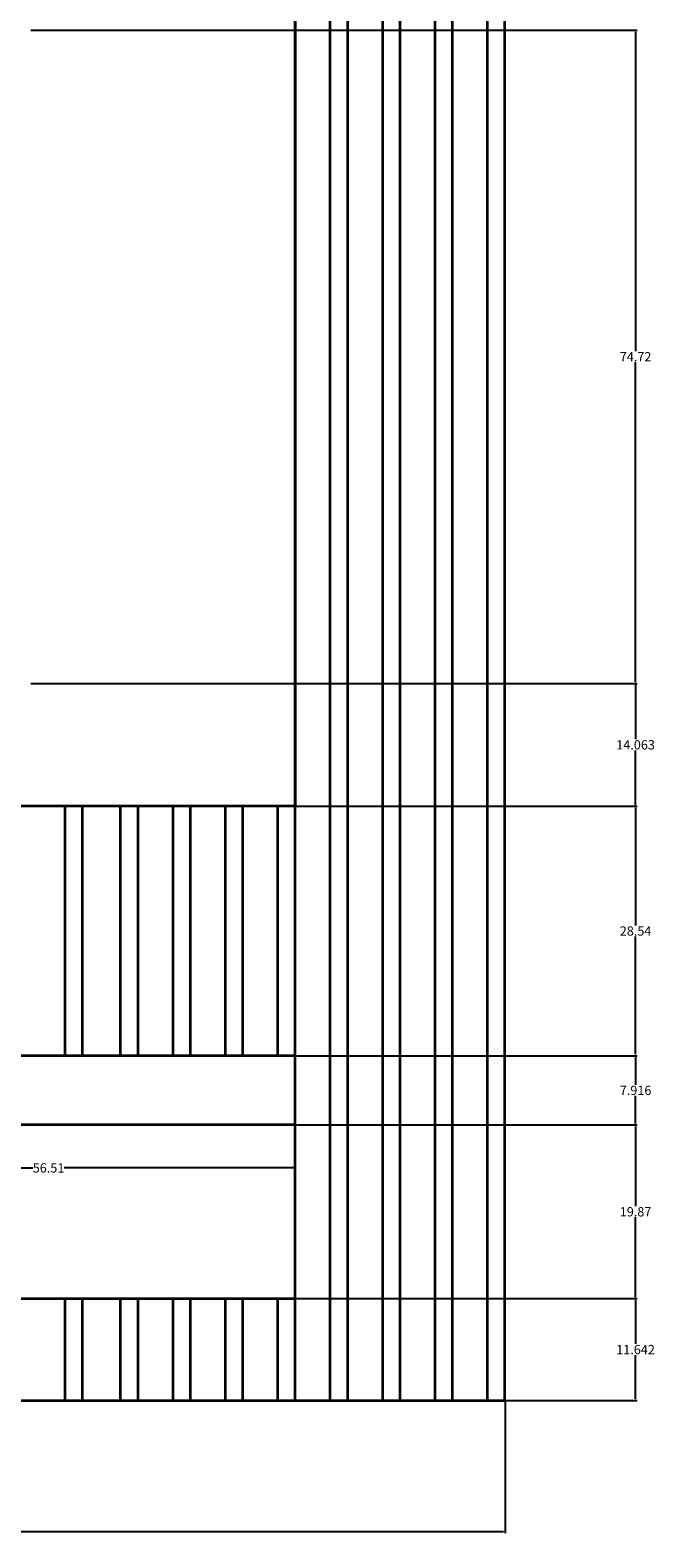
# Model space of a CAD drawing. Units: inches. Extents: x 35 to 365, y 67 to 380.
# Tile 4 of 5: x 293 to 365, y 67 to 240. Entities that reach past the tile are written whole.
import ezdxf

# ---------------------------------------------------------------- set-up
doc = ezdxf.new("R2010")
doc.units = ezdxf.units.IN
doc.header["$MEASUREMENT"] = 0
doc.layers.add('A-ANNO-DIMS', color=2, linetype='Continuous', lineweight=18)
doc.layers.add('A-FURN', color=7, linetype='Continuous', lineweight=35)
doc.styles.get("Standard").update_dxf_attribs({"font": 'arial.ttf'})
doc.dimstyles.get("Standard").update_dxf_attribs({"dimtxt": 1.0625, "dimasz": 0.18, "dimexe": 0.18, "dimexo": 0.0625, "dimgap": 0.09, "dimtad": 0, "dimtih": 1, "dimtoh": 1, "dimdec": 4, "dimzin": 0, "dimdsep": 46, "dimlunit": 4, "dimtxsty": 'Standard', "dimcen": 0.09, "dimadec": 0, "dimazin": 0, "dimtfac": 1, "dimtdec": 4, "dimtofl": 0, "dimtmove": 0, "dimatfit": 3, "dimfxl": 1, "dimtolj": 1, "dimtzin": 0, "dimarcsym": 0})

# ---------------------------------------------------------------- blocks, each defined once
blk = doc.blocks.new('*D9')
at = {"layer": 'A-ANNO-DIMS', "color": 0, "lineweight": -2, "transparency": 16777216}
for p, q in [((51.28, 94.63), (51.28, 67.85)), ((347.67, 82.99), (347.67, 67.85)), ((51.46, 68.03), (197.58, 68.03)), ((347.49, 68.03), (201.36, 68.03))]:
    blk.add_line(p, q, dxfattribs=at)
at = {"layer": 'A-ANNO-DIMS', "color": 0, "transparency": 16777216}
for points in [[(51.46, 68.06), (51.46, 68), (51.28, 68.03)], [(347.49, 68.06), (347.49, 68), (347.67, 68.03)]]:
    blk.add_solid(points, dxfattribs=at)
at = {"layer": 'Defpoints', "color": 0, "transparency": 16777216}
for p in [(51.28, 94.7), (347.67, 83.05), (347.67, 68.03)]:
    blk.add_point(p, dxfattribs=at)
at = {"layer": 'A-ANNO-DIMS', "color": 0, "transparency": 16777216, "insert": (199.47, 68.03), "char_height": 1.062, "attachment_point": 5}
blk.add_mtext('\\A1;296.4', dxfattribs=at)
blk = doc.blocks.new('*D20')
at = {"layer": 'A-ANNO-DIMS', "color": 0, "lineweight": -2, "transparency": 16777216}
for p, q in [((267.16, 94.76), (267.16, 109.83)), ((267.34, 109.65), (293.63, 109.65)), ((323.49, 109.65), (297.19, 109.65)), ((323.67, 94.76), (323.67, 109.83))]:
    blk.add_line(p, q, dxfattribs=at)
at = {"layer": 'A-ANNO-DIMS', "color": 0, "transparency": 16777216}
for points in [[(267.34, 109.68), (267.34, 109.62), (267.16, 109.65)], [(323.49, 109.68), (323.49, 109.62), (323.67, 109.65)]]:
    blk.add_solid(points, dxfattribs=at)
at = {"layer": 'Defpoints', "color": 0, "transparency": 16777216}
for p in [(323.67, 109.65), (267.16, 94.7), (323.67, 94.7)]:
    blk.add_point(p, dxfattribs=at)
at = {"layer": 'A-ANNO-DIMS', "color": 0, "transparency": 16777216, "insert": (295.41, 109.65), "char_height": 1.062, "attachment_point": 5}
blk.add_mtext('\\A1;56.51', dxfattribs=at)
blk = doc.blocks.new('*D21')
at = {"layer": 'A-ANNO-DIMS', "color": 0, "lineweight": -2, "transparency": 16777216}
for p, q in [((323.73, 94.7), (362.8, 94.7)), ((362.62, 94.52), (362.62, 89.51)), ((362.62, 83.23), (362.62, 88.24)), ((347.73, 83.05), (362.8, 83.05))]:
    blk.add_line(p, q, dxfattribs=at)
at = {"layer": 'A-ANNO-DIMS', "color": 0, "transparency": 16777216}
for points in [[(362.59, 94.52), (362.65, 94.52), (362.62, 94.7)], [(362.59, 83.23), (362.65, 83.23), (362.62, 83.05)]]:
    blk.add_solid(points, dxfattribs=at)
at = {"layer": 'Defpoints', "color": 0, "transparency": 16777216}
for p in [(323.67, 94.7), (362.62, 94.7), (347.67, 83.05)]:
    blk.add_point(p, dxfattribs=at)
at = {"layer": 'A-ANNO-DIMS', "color": 0, "transparency": 16777216, "insert": (362.62, 88.87), "char_height": 1.062, "attachment_point": 5}
blk.add_mtext('\\A1;11.642', dxfattribs=at)
blk = doc.blocks.new('*D22')
at = {"layer": 'A-ANNO-DIMS', "color": 0, "lineweight": -2, "transparency": 16777216}
for p, q in [((323.73, 114.56), (362.8, 114.56)), ((362.62, 114.38), (362.62, 105.26)), ((362.62, 94.88), (362.62, 104)), ((323.73, 94.7), (362.8, 94.7))]:
    blk.add_line(p, q, dxfattribs=at)
at = {"layer": 'A-ANNO-DIMS', "color": 0, "transparency": 16777216}
for points in [[(362.59, 114.38), (362.65, 114.38), (362.62, 114.56)], [(362.59, 94.88), (362.65, 94.88), (362.62, 94.7)]]:
    blk.add_solid(points, dxfattribs=at)
at = {"layer": 'Defpoints', "color": 0, "transparency": 16777216}
for p in [(323.67, 114.56), (362.62, 114.56), (323.67, 94.7)]:
    blk.add_point(p, dxfattribs=at)
at = {"layer": 'A-ANNO-DIMS', "color": 0, "transparency": 16777216, "insert": (362.62, 104.63), "char_height": 1.062, "attachment_point": 5}
blk.add_mtext('\\A1;19.87', dxfattribs=at)
blk = doc.blocks.new('*D23')
at = {"layer": 'A-ANNO-DIMS', "color": 0, "lineweight": -2, "transparency": 16777216}
for p, q in [((323.73, 122.48), (362.8, 122.48)), ((362.62, 122.3), (362.62, 119.16)), ((362.62, 114.74), (362.62, 117.89)), ((323.73, 114.56), (362.8, 114.56))]:
    blk.add_line(p, q, dxfattribs=at)
at = {"layer": 'A-ANNO-DIMS', "color": 0, "transparency": 16777216}
for points in [[(362.59, 122.3), (362.65, 122.3), (362.62, 122.48)], [(362.59, 114.74), (362.65, 114.74), (362.62, 114.56)]]:
    blk.add_solid(points, dxfattribs=at)
at = {"layer": 'Defpoints', "color": 0, "transparency": 16777216}
for p in [(323.67, 122.48), (362.62, 122.48), (323.67, 114.56)]:
    blk.add_point(p, dxfattribs=at)
at = {"layer": 'A-ANNO-DIMS', "color": 0, "transparency": 16777216, "insert": (362.62, 118.52), "char_height": 1.062, "attachment_point": 5}
blk.add_mtext('\\A1;7.916', dxfattribs=at)
blk = doc.blocks.new('*D24')
at = {"layer": 'A-ANNO-DIMS', "color": 0, "lineweight": -2, "transparency": 16777216}
for p, q in [((323.73, 151.02), (362.8, 151.02)), ((362.62, 150.84), (362.62, 137.38)), ((362.62, 122.66), (362.62, 136.12)), ((323.73, 122.48), (362.8, 122.48))]:
    blk.add_line(p, q, dxfattribs=at)
at = {"layer": 'A-ANNO-DIMS', "color": 0, "transparency": 16777216}
for points in [[(362.59, 150.84), (362.65, 150.84), (362.62, 151.02)], [(362.59, 122.66), (362.65, 122.66), (362.62, 122.48)]]:
    blk.add_solid(points, dxfattribs=at)
at = {"layer": 'Defpoints', "color": 0, "transparency": 16777216}
for p in [(323.67, 151.02), (362.62, 151.02), (323.67, 122.48)]:
    blk.add_point(p, dxfattribs=at)
at = {"layer": 'A-ANNO-DIMS', "color": 0, "transparency": 16777216, "insert": (362.62, 136.75), "char_height": 1.062, "attachment_point": 5}
blk.add_mtext('\\A1;28.54', dxfattribs=at)
blk = doc.blocks.new('*D25')
at = {"layer": 'A-ANNO-DIMS', "color": 0, "lineweight": -2, "transparency": 16777216}
for p, q in [((293.37, 165.08), (362.8, 165.08)), ((362.62, 164.9), (362.62, 158.68)), ((362.62, 151.2), (362.62, 157.42)), ((323.73, 151.02), (362.8, 151.02))]:
    blk.add_line(p, q, dxfattribs=at)
at = {"layer": 'A-ANNO-DIMS', "color": 0, "transparency": 16777216}
for points in [[(362.59, 164.9), (362.65, 164.9), (362.62, 165.08)], [(362.59, 151.2), (362.65, 151.2), (362.62, 151.02)]]:
    blk.add_solid(points, dxfattribs=at)
at = {"layer": 'Defpoints', "color": 0, "transparency": 16777216}
for p in [(293.3, 165.08), (362.62, 165.08), (323.67, 151.02)]:
    blk.add_point(p, dxfattribs=at)
at = {"layer": 'A-ANNO-DIMS', "color": 0, "transparency": 16777216, "insert": (362.62, 158.05), "char_height": 1.062, "attachment_point": 5}
blk.add_mtext('\\A1;14.063', dxfattribs=at)
blk = doc.blocks.new('*D26')
at = {"layer": 'A-ANNO-DIMS', "color": 0, "lineweight": -2, "transparency": 16777216}
for p, q in [((293.37, 239.81), (362.8, 239.81)), ((362.62, 239.63), (362.62, 203.07)), ((362.62, 165.26), (362.62, 201.82)), ((293.37, 165.08), (362.8, 165.08))]:
    blk.add_line(p, q, dxfattribs=at)
at = {"layer": 'A-ANNO-DIMS', "color": 0, "transparency": 16777216}
for points in [[(362.59, 239.63), (362.65, 239.63), (362.62, 239.81)], [(362.59, 165.26), (362.65, 165.26), (362.62, 165.08)]]:
    blk.add_solid(points, dxfattribs=at)
at = {"layer": 'Defpoints', "color": 0, "transparency": 16777216}
for p in [(293.3, 239.81), (362.62, 239.81), (293.3, 165.08)]:
    blk.add_point(p, dxfattribs=at)
at = {"layer": 'A-ANNO-DIMS', "color": 0, "transparency": 16777216, "insert": (362.62, 202.45), "char_height": 1.062, "attachment_point": 5}
blk.add_mtext('\\A1;74.72', dxfattribs=at)

msp = doc.modelspace()

# ---------------------------------------------------------------- linework, layer by layer
at = {"layer": 'A-FURN'}
for p, q in [((323.6655, 82.9768), (323.6655, 293.4266)), ((327.6655, 82.9768), (327.6655, 293.4266)), ((329.6655, 82.9768), (329.6655, 293.4266)), ((333.6655, 82.9768), (333.6655, 293.4266)), ((335.6655, 82.9768), (335.6655, 293.4266)), ((339.6655, 82.9768), (339.6655, 293.4266)), ((341.6655, 82.9768), (341.6655, 293.4266)), ((345.6655, 83.0529), (345.6655, 293.5027)), ((347.6655, 83.0529), (347.6655, 293.5027)), ((297.3029, 122.4805), (297.3029, 151.0198)), ((299.3029, 122.4805), (299.3029, 151.0198)), ((303.6655, 122.4805), (303.6655, 151.0198)), ((305.6655, 122.4805), (305.6655, 151.0198)), ((309.6655, 122.4805), (309.6655, 151.0198)), ((311.6655, 122.4805), (311.6655, 151.0198)), ((315.6655, 122.4805), (315.6655, 151.0198)), ((317.6655, 122.4805), (317.6655, 151.0198)), ((321.6655, 122.4805), (321.6655, 151.0198)), ((323.6655, 122.4805), (115.383, 122.4805)), ((323.6655, 114.5646), (323.6655, 122.4805)), ((323.6655, 114.5646), (51.2797, 114.5646)), ((323.6655, 94.6954), (323.6655, 114.5646)), ((51.2797, 94.6954), (323.6655, 94.6954)), ((297.3029, 82.9768), (297.3029, 94.6954)), ((299.3029, 82.9768), (299.3029, 94.6954)), ((303.6655, 82.9768), (303.6655, 94.6954)), ((305.6655, 82.9768), (305.6655, 94.6954)), ((309.6655, 82.9768), (309.6655, 94.6954)), ((311.6655, 82.9768), (311.6655, 94.6954)), ((315.6655, 82.9768), (315.6655, 94.6954)), ((317.6655, 82.9768), (317.6655, 94.6954)), ((321.6655, 82.9768), (321.6655, 94.6954)), ((61.3227, 83.0529), (347.6655, 83.0529))]:
    msp.add_line(p, q, dxfattribs=at)
msp.add_lwpolyline([(115.383, 254.0695), (323.6655, 254.0695), (323.6655, 151.0198), (115.383, 151.0198)], close=True, dxfattribs=at)

# ---------------------------------------------------------------- dimensions: what is measured, and where the dimension line sits
at = {"layer": 'A-ANNO-DIMS'}
for base, p1, p2, override, picture, middle in [((362.6155, 239.8076), (293.3029, 165.0829), (293.3029, 239.8076), {"dimdec": 2, "dimlfac": 1, "dimrnd": 0, "dimzin": 0, "dimdsep": 46, "dimlunit": 2}, '*D26', (362.6155, 202.4453)), ((362.6155, 165.0829), (323.6655, 151.0198), (293.3029, 165.0829), {"dimdec": 3, "dimlfac": 1, "dimrnd": 0, "dimzin": 0, "dimdsep": 46, "dimlunit": 2}, '*D25', (362.6155, 158.0514)), ((362.6155, 151.0198), (323.6655, 122.4805), (323.6655, 151.0198), {"dimdec": 2, "dimlfac": 1, "dimrnd": 0, "dimzin": 0, "dimdsep": 46, "dimlunit": 2}, '*D24', (362.6155, 136.7502)), ((362.6155, 122.4805), (323.6655, 114.5646), (323.6655, 122.4805), {"dimdec": 3, "dimlfac": 1, "dimrnd": 0, "dimzin": 0, "dimdsep": 46, "dimlunit": 2}, '*D23', (362.6155, 118.5226)), ((362.6155, 114.5646), (323.6655, 94.6954), (323.6655, 114.5646), {"dimdec": 2, "dimlfac": 1, "dimrnd": 0, "dimzin": 0, "dimdsep": 46, "dimlunit": 2}, '*D22', (362.6155, 104.63)), ((362.61553, 94.69536), (347.66553, 83.05291), (323.66553, 94.69536), {"dimdec": 3, "dimlfac": 1, "dimrnd": 0, "dimzin": 0, "dimdsep": 46, "dimlunit": 2}, '*D21', (362.61553, 88.87414))]:
    dim = msp.add_linear_dim(base=base, p1=p1, p2=p2, angle=90, dimstyle='Standard', override=override, dxfattribs=at)
    dim.commit()
    dim.dimension.update_dxf_attribs({"geometry": picture, "text_midpoint": middle})
for base, p1, p2, override, picture, middle in [((323.6655, 109.6454), (267.1558, 94.6954), (323.6655, 94.6954), {"dimdec": 2, "dimlfac": 1, "dimrnd": 0, "dimzin": 0, "dimdsep": 46, "dimlunit": 2}, '*D20', (295.4107, 109.6454)), ((347.6655, 68.0268), (51.2797, 94.6954), (347.6655, 83.0529), {"dimdec": 1, "dimlfac": 1, "dimrnd": 0, "dimzin": 0, "dimdsep": 46, "dimlunit": 2}, '*D9', (199.4726, 68.0268))]:
    dim = msp.add_linear_dim(base=base, p1=p1, p2=p2, dimstyle='Standard', override=override, dxfattribs=at)
    dim.commit()
    dim.dimension.update_dxf_attribs({"geometry": picture, "text_midpoint": middle})

doc.saveas('drawing.dxf')
